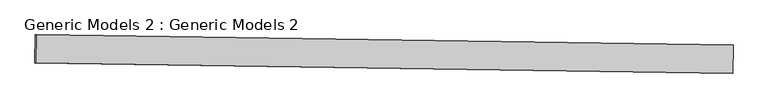
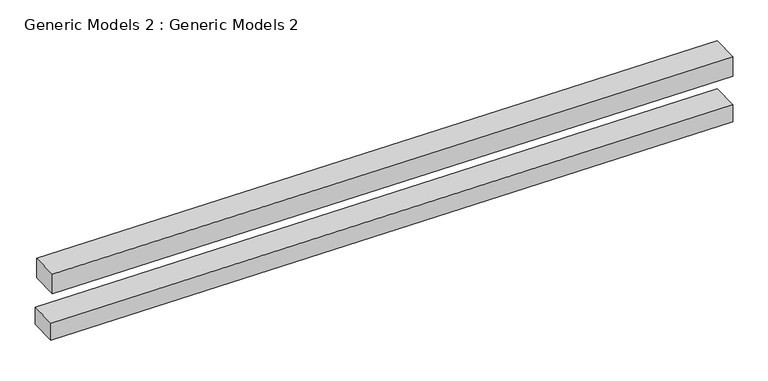
"""IFC4 building model written with IfcOpenShell, lengths in millimetres: proxy geometry, Generic Models 2 : Generic Models 2."""

from ifc_helpers import new_model, si_unit, frame, origin, place, context, project, spatial, polyline, outline, extrude, source, transform, mapped, element, save


def generic_models_2_generic_models_2_96ab2cd9(model_context):
    return source(origin(), model_context, "Body", "SweptSolid", [
        extrude(outline(polyline([(7680.1321867, -8736.7927893), (210.5189509, -8627.4051351), (214.9820712, -8322.6378131), (7684.595307, -8432.0254673), (7680.1321867, -8736.7927893)])), frame((0.0, 0.0, 674.6370613), z_axis=(0.0, 0.0, 1.0), x_axis=(1.0, 0.0, 0.0)), (0.0, 0.0, 1.0), 229.727366),
        extrude(outline(polyline([(7680.1321867, -8736.7927893), (193.8246586, -8627.160658), (198.2877789, -8322.393336), (7684.595307, -8432.0254673), (7680.1321867, -8736.7927893)])), frame((0.0, 0.0, 138.9068149), z_axis=(0.0, 0.0, 1.0), x_axis=(1.0, 0.0, 0.0)), (0.0, 0.0, 1.0), 199.5053968),
    ])


if __name__ == "__main__":
    model = new_model("IFC4")
    model_context = context("Model", 3, world=origin())
    ifc_project = project(units=[si_unit("LENGTHUNIT", "METRE", prefix="MILLI")], contexts=[model_context])
    site = spatial("IfcSite", under=ifc_project)
    building = spatial("IfcBuilding", under=site)
    placement = place(None, origin())
    generic_models_2_generic_models_2_shape = generic_models_2_generic_models_2_96ab2cd9(model_context)
    element("IfcBuildingElementProxy", 1, Name="Generic Models 2 : Generic Models 2", ObjectType="Generic Models 2 : Generic Models 2", at=placement, inside=building, context=model_context, shape_type="MappedRepresentation", body=[
        mapped(generic_models_2_generic_models_2_shape, transform((0.0, 0.0, 0.0), x_axis=(1.0, 0.0, 0.0), y_axis=(0.0, 1.0, 0.0), z_axis=(0.0, 0.0, 1.0))),
    ])
    save(model, "model.ifc")

# Revit data of these elements
# Element 1 (IfcBuildingElementProxy, "Generic Models 2 : Generic Models 2")
#   Materials on its faces: "Parking Stripe"
# Materials
#   "Parking Stripe": class "Paint", colour RGB 250 250 91, transparency 0, Cost = 0
